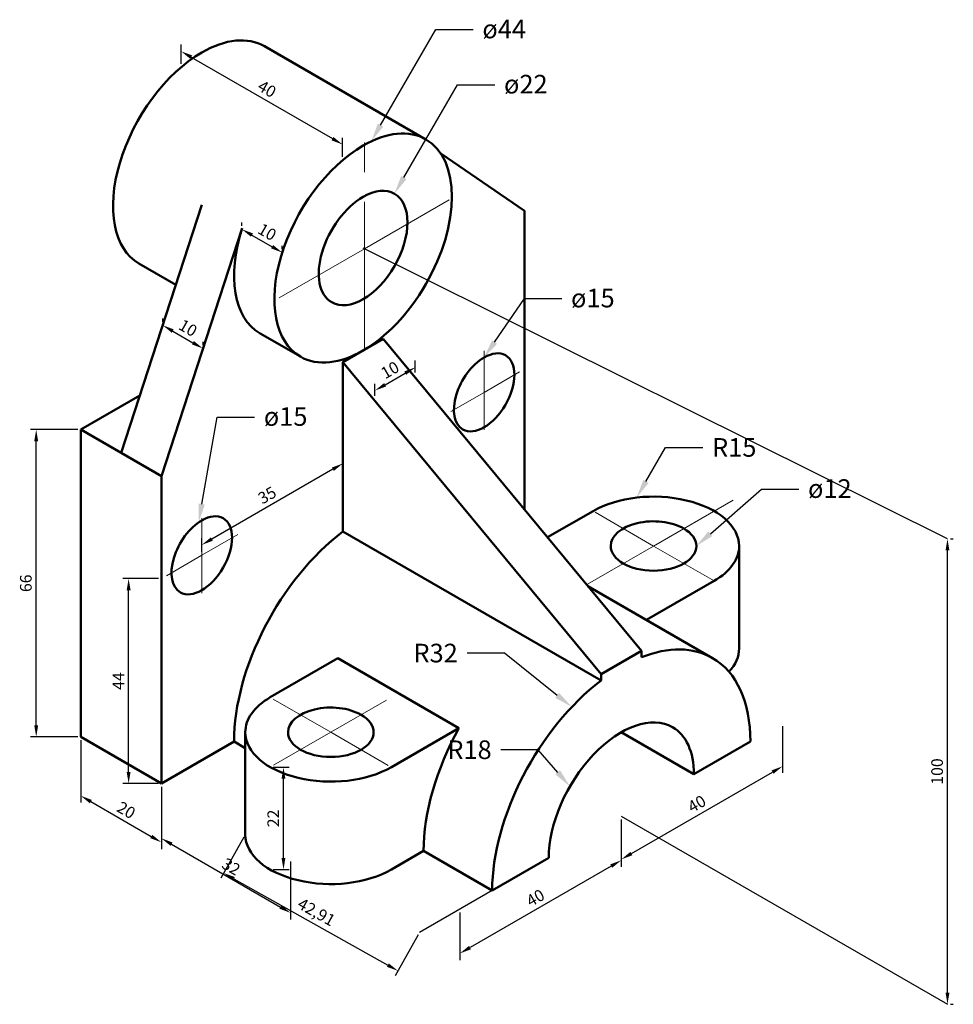
# Model space of a CAD drawing. Units: millimetres. Extents: x 3050 to 3251, y 1794 to 2006.
import ezdxf
from ezdxf import colors
from ezdxf.entities.mleader import LeaderData, LeaderLine
from ezdxf.math import Vec2, Vec3

# ---------------------------------------------------------------- set-up
doc = ezdxf.new("R2010")
doc.units = ezdxf.units.MM
doc.linetypes.add('CENTER', pattern=[50.8, 31.75, -6.35, 6.35, -6.35])
for name, color, linetype, lineweight in [('M-CNTR', 1, 'CENTER', 18), ('M-DIMS', 2, 'Continuous', 25), ('M-OUTL', 7, 'Continuous', 50), ('M-TEXT', 3, 'Continuous', 25)]:
    doc.layers.add(name, color=color, linetype=linetype, lineweight=lineweight)
doc.styles.get("Standard").update_dxf_attribs({"font": 'arial.ttf'})
doc.dimstyles.new('ISO-25', dxfattribs={"dimtxt": 2.5, "dimasz": 2.5, "dimexe": 1.25, "dimexo": 0.625, "dimtad": 1, "dimtxsty": 'Standard', "dimcen": 2.5, "dimadec": 0, "dimazin": 0, "dimtfac": 1, "dimtmove": 0, "dimatfit": 3, "dimfxl": 1, "dimarcsym": 0})

# ---------------------------------------------------------------- blocks, each defined once
blk = doc.blocks.new('*D1')
at = {"layer": 'Defpoints', "color": 0, "transparency": 16777216}
for p in [(3063.23, 1851.76), (3080.55, 1841.76), (3080.55, 1829.12)]:
    blk.add_point(p, dxfattribs=at)
at = {"layer": 'M-DIMS', "color": 0, "lineweight": -2, "transparency": 16777216}
for p, q in [((3063.23, 1851.04), (3063.23, 1837.67)), ((3080.55, 1841.04), (3080.55, 1827.67)), ((3065.39, 1837.87), (3078.38, 1830.37))]:
    blk.add_line(p, q, dxfattribs=at)
at = {"layer": 'M-DIMS', "color": 0, "transparency": 16777216}
for points in [[(3065.6, 1838.23), (3065.18, 1837.51), (3063.23, 1839.12)], [(3078.59, 1830.73), (3078.18, 1830.01), (3080.55, 1829.12)]]:
    blk.add_solid(points, dxfattribs=at)
at = {"layer": 'M-DIMS', "color": 0, "transparency": 16777216, "insert": (3072.84, 1835.76), "char_height": 2.5, "attachment_point": 5, "rotation": 330}
blk.add_mtext('20', dxfattribs=at)
blk = doc.blocks.new('*D2')
at = {"layer": 'Defpoints', "color": 0, "transparency": 16777216}
for p in [(3080.55, 1841.76), (3108.26, 1825.76), (3108.26, 1813.98)]:
    blk.add_point(p, dxfattribs=at)
at = {"layer": 'M-DIMS', "color": 0, "lineweight": -2, "transparency": 16777216}
for p, q in [((3080.55, 1841.04), (3080.55, 1828.54)), ((3082.71, 1828.73), (3106.1, 1815.23)), ((3108.26, 1825.04), (3108.26, 1812.54))]:
    blk.add_line(p, q, dxfattribs=at)
at = {"layer": 'M-DIMS', "color": 0, "transparency": 16777216}
for points in [[(3082.92, 1829.09), (3082.51, 1828.37), (3080.55, 1829.98)], [(3106.3, 1815.59), (3105.89, 1814.87), (3108.26, 1813.98)]]:
    blk.add_solid(points, dxfattribs=at)
at = {"layer": 'M-DIMS', "color": 0, "transparency": 16777216, "insert": (3095.36, 1823.63), "char_height": 2.5, "attachment_point": 5, "rotation": 330}
blk.add_mtext('32', dxfattribs=at)
blk = doc.blocks.new('*D3')
at = {"layer": 'Defpoints', "color": 0, "transparency": 16777216}
for p in [(3179.28, 1834.76), (3144.63, 1814.76), (3144.63, 1805.27)]:
    blk.add_point(p, dxfattribs=at)
at = {"layer": 'M-DIMS', "color": 0, "lineweight": -2, "transparency": 16777216}
for p, q in [((3179.28, 1834.04), (3179.28, 1823.83)), ((3177.11, 1824.02), (3146.8, 1806.52)), ((3144.63, 1814.04), (3144.63, 1803.83))]:
    blk.add_line(p, q, dxfattribs=at)
at = {"layer": 'M-DIMS', "color": 0, "transparency": 16777216}
for points in [[(3176.9, 1824.38), (3177.32, 1823.66), (3179.28, 1825.27)], [(3146.59, 1806.88), (3147.01, 1806.16), (3144.63, 1805.27)]]:
    blk.add_solid(points, dxfattribs=at)
at = {"layer": 'M-DIMS', "color": 0, "transparency": 16777216, "insert": (3161, 1816.92), "char_height": 2.5, "attachment_point": 5, "rotation": 30}
blk.add_mtext('40', dxfattribs=at)
blk = doc.blocks.new('*D4')
at = {"layer": 'Defpoints', "color": 0, "transparency": 16777216}
for p in [(3213.92, 1854.76), (3213.92, 1845.46), (3179.28, 1834.76)]:
    blk.add_point(p, dxfattribs=at)
at = {"layer": 'M-DIMS', "color": 0, "lineweight": -2, "transparency": 16777216}
for p, q in [((3213.92, 1854.04), (3213.92, 1844.02)), ((3181.44, 1826.71), (3211.75, 1844.21)), ((3179.28, 1834.04), (3179.28, 1824.02))]:
    blk.add_line(p, q, dxfattribs=at)
at = {"layer": 'M-DIMS', "color": 0, "transparency": 16777216}
for points in [[(3211.54, 1844.57), (3211.96, 1843.85), (3213.92, 1845.46)], [(3181.23, 1827.07), (3181.65, 1826.35), (3179.28, 1825.46)]]:
    blk.add_solid(points, dxfattribs=at)
at = {"layer": 'M-DIMS', "color": 0, "transparency": 16777216, "insert": (3195.65, 1837.11), "char_height": 2.5, "attachment_point": 5, "rotation": 30}
blk.add_mtext('40', dxfattribs=at)
blk = doc.blocks.new('*D5')
at = {"layer": 'Defpoints', "color": 0, "transparency": 16777216}
for p in [(3053.67, 1917.76), (3063.23, 1917.76), (3063.23, 1851.76)]:
    blk.add_point(p, dxfattribs=at)
at = {"layer": 'M-DIMS', "color": 0, "lineweight": -2, "transparency": 16777216}
for p, q in [((3062.6, 1917.76), (3052.42, 1917.76)), ((3053.67, 1854.26), (3053.67, 1915.26)), ((3062.6, 1851.76), (3052.42, 1851.76))]:
    blk.add_line(p, q, dxfattribs=at)
at = {"layer": 'M-DIMS', "color": 0, "transparency": 16777216}
for points in [[(3053.25, 1915.26), (3054.09, 1915.26), (3053.67, 1917.76)], [(3053.25, 1854.26), (3054.09, 1854.26), (3053.67, 1851.76)]]:
    blk.add_solid(points, dxfattribs=at)
at = {"layer": 'M-DIMS', "color": 0, "transparency": 16777216, "insert": (3051.77, 1884.76), "char_height": 2.5, "attachment_point": 5, "rotation": 90}
blk.add_mtext('66', dxfattribs=at)
blk = doc.blocks.new('*D6')
at = {"layer": 'Defpoints', "color": 0, "transparency": 16777216}
for p in [(3073.51, 1885.76), (3080.55, 1885.76), (3080.55, 1841.76)]:
    blk.add_point(p, dxfattribs=at)
at = {"layer": 'M-DIMS', "color": 0, "lineweight": -2, "transparency": 16777216}
for p, q in [((3079.92, 1885.76), (3072.26, 1885.76)), ((3073.51, 1844.26), (3073.51, 1883.26)), ((3079.92, 1841.76), (3072.26, 1841.76))]:
    blk.add_line(p, q, dxfattribs=at)
at = {"layer": 'M-DIMS', "color": 0, "transparency": 16777216}
for points in [[(3073.09, 1883.26), (3073.93, 1883.26), (3073.51, 1885.76)], [(3073.09, 1844.26), (3073.93, 1844.26), (3073.51, 1841.76)]]:
    blk.add_solid(points, dxfattribs=at)
at = {"layer": 'M-DIMS', "color": 0, "transparency": 16777216, "insert": (3071.64, 1863.76), "char_height": 2.5, "attachment_point": 5, "rotation": 90}
blk.add_mtext('44', dxfattribs=at)
blk = doc.blocks.new('*D7')
at = {"layer": 'Defpoints', "color": 0, "transparency": 16777216}
for p in [(3119.52, 1908.26), (3089.21, 1893), (3089.21, 1890.76)]:
    blk.add_point(p, dxfattribs=at)
at = {"layer": 'M-DIMS', "color": 0, "lineweight": -2, "transparency": 16777216}
for p, q in [((3119.52, 1908.99), (3119.52, 1911.95)), ((3117.35, 1909.25), (3091.37, 1894.25)), ((3089.21, 1891.49), (3089.21, 1894.45))]:
    blk.add_line(p, q, dxfattribs=at)
at = {"layer": 'M-DIMS', "color": 0, "transparency": 16777216}
for points in [[(3117.15, 1909.61), (3117.56, 1908.89), (3119.52, 1910.5)], [(3091.17, 1894.61), (3091.58, 1893.89), (3089.21, 1893)]]:
    blk.add_solid(points, dxfattribs=at)
at = {"layer": 'M-DIMS', "color": 0, "transparency": 16777216, "insert": (3103.41, 1903.4), "char_height": 2.5, "attachment_point": 5, "rotation": 30}
blk.add_mtext('35', dxfattribs=at)
blk = doc.blocks.new('*D8')
at = {"layer": 'Defpoints', "color": 0, "transparency": 16777216}
for p in [(3135.06, 1931.15), (3135.06, 1929.33), (3126.4, 1924.33)]:
    blk.add_point(p, dxfattribs=at)
at = {"layer": 'M-DIMS', "color": 0, "lineweight": -2, "transparency": 16777216}
for p, q in [((3135.06, 1930.05), (3135.06, 1932.59)), ((3128.57, 1927.4), (3132.9, 1929.9)), ((3126.4, 1925.05), (3126.4, 1927.59))]:
    blk.add_line(p, q, dxfattribs=at)
at = {"layer": 'M-DIMS', "color": 0, "transparency": 16777216}
for points in [[(3132.69, 1930.26), (3133.1, 1929.53), (3135.06, 1931.15)], [(3128.36, 1927.76), (3128.77, 1927.03), (3126.4, 1926.15)]]:
    blk.add_solid(points, dxfattribs=at)
at = {"layer": 'M-DIMS', "color": 0, "transparency": 16777216, "insert": (3129.78, 1930.29), "char_height": 2.5, "attachment_point": 5, "rotation": 30}
blk.add_mtext('10', dxfattribs=at)
blk = doc.blocks.new('*D9')
at = {"layer": 'Defpoints', "color": 0, "transparency": 16777216}
for p in [(3103.93, 1845.26), (3106.76, 1845.26), (3103.93, 1823.26)]:
    blk.add_point(p, dxfattribs=at)
at = {"layer": 'M-DIMS', "color": 0, "lineweight": -2, "transparency": 16777216}
for p, q in [((3104.56, 1845.26), (3108.01, 1845.26)), ((3106.76, 1825.76), (3106.76, 1842.76)), ((3104.56, 1823.26), (3108.01, 1823.26))]:
    blk.add_line(p, q, dxfattribs=at)
at = {"layer": 'M-DIMS', "color": 0, "transparency": 16777216}
for points in [[(3106.34, 1842.76), (3107.17, 1842.76), (3106.76, 1845.26)], [(3106.34, 1825.76), (3107.17, 1825.76), (3106.76, 1823.26)]]:
    blk.add_solid(points, dxfattribs=at)
at = {"layer": 'M-DIMS', "color": 0, "transparency": 16777216, "insert": (3104.88, 1834.26), "char_height": 2.5, "attachment_point": 5, "rotation": 90}
blk.add_mtext('22', dxfattribs=at)
blk = doc.blocks.new('*D10')
at = {"layer": 'Defpoints', "color": 0, "transparency": 16777216}
for p in [(3080.82, 1940.18), (3089.48, 1935.18), (3089.48, 1935.18)]:
    blk.add_point(p, dxfattribs=at)
at = {"layer": 'M-DIMS', "color": 0, "lineweight": -2, "transparency": 16777216}
for p, q in [((3080.82, 1940.9), (3080.82, 1941.62)), ((3082.98, 1938.93), (3087.31, 1936.43)), ((3089.48, 1935.9), (3089.48, 1936.62))]:
    blk.add_line(p, q, dxfattribs=at)
at = {"layer": 'M-DIMS', "color": 0, "transparency": 16777216}
for points in [[(3083.19, 1939.29), (3082.78, 1938.56), (3080.82, 1940.18)], [(3087.52, 1936.79), (3087.11, 1936.06), (3089.48, 1935.18)]]:
    blk.add_solid(points, dxfattribs=at)
at = {"layer": 'M-DIMS', "color": 0, "transparency": 16777216, "insert": (3086.1, 1939.32), "char_height": 2.5, "attachment_point": 5, "rotation": 330}
blk.add_mtext('10', dxfattribs=at)
blk = doc.blocks.new('*D11')
at = {"layer": 'Defpoints', "color": 0, "transparency": 16777216}
for p in [(3097.82, 1960.79), (3106.48, 1955.79), (3106.48, 1955.79)]:
    blk.add_point(p, dxfattribs=at)
at = {"layer": 'M-DIMS', "color": 0, "lineweight": -2, "transparency": 16777216}
for p, q in [((3097.82, 1961.51), (3097.82, 1962.23)), ((3099.99, 1959.54), (3104.32, 1957.04)), ((3106.48, 1956.51), (3106.48, 1957.23))]:
    blk.add_line(p, q, dxfattribs=at)
at = {"layer": 'M-DIMS', "color": 0, "transparency": 16777216}
for points in [[(3100.2, 1959.9), (3099.78, 1959.18), (3097.82, 1960.79)], [(3104.53, 1957.4), (3104.11, 1956.68), (3106.48, 1955.79)]]:
    blk.add_solid(points, dxfattribs=at)
at = {"layer": 'M-DIMS', "color": 0, "transparency": 16777216, "insert": (3103.1, 1959.93), "char_height": 2.5, "attachment_point": 5, "rotation": 330}
blk.add_mtext('10', dxfattribs=at)
blk = doc.blocks.new('*D12')
at = {"layer": 'Defpoints', "color": 0, "transparency": 16777216}
for p in [(3084.79, 1995.61), (3119.43, 1979), (3119.43, 1975.61)]:
    blk.add_point(p, dxfattribs=at)
at = {"layer": 'M-DIMS', "color": 0, "lineweight": -2, "transparency": 16777216}
for p, q in [((3084.79, 1996.34), (3084.79, 2000.45)), ((3086.95, 1997.75), (3117.27, 1980.25)), ((3119.43, 1976.34), (3119.43, 1980.45))]:
    blk.add_line(p, q, dxfattribs=at)
at = {"layer": 'M-DIMS', "color": 0, "transparency": 16777216}
for points in [[(3087.16, 1998.12), (3086.75, 1997.39), (3084.79, 1999)], [(3117.47, 1980.62), (3117.06, 1979.89), (3119.43, 1979)]]:
    blk.add_solid(points, dxfattribs=at)
at = {"layer": 'M-DIMS', "color": 0, "transparency": 16777216, "insert": (3103.06, 1990.65), "char_height": 2.5, "attachment_point": 5, "rotation": 330}
blk.add_mtext('40', dxfattribs=at)
blk = doc.blocks.new('*D13')
at = {"layer": 'Defpoints', "color": 0, "transparency": 16777216}
for p in [(3098.55, 1830.76), (3135.97, 1809.76), (3131.35, 1801.52)]:
    blk.add_point(p, dxfattribs=at)
at = {"layer": 'M-DIMS', "color": 0, "lineweight": -2, "transparency": 16777216}
for p, q in [((3098.24, 1830.22), (3093.32, 1821.43)), ((3096.11, 1821.3), (3129.17, 1802.75)), ((3135.67, 1809.22), (3130.74, 1800.43))]:
    blk.add_line(p, q, dxfattribs=at)
at = {"layer": 'M-DIMS', "color": 0, "transparency": 16777216}
for points in [[(3096.31, 1821.66), (3095.9, 1820.94), (3093.93, 1822.52)], [(3129.37, 1803.11), (3128.97, 1802.38), (3131.35, 1801.52)]]:
    blk.add_solid(points, dxfattribs=at)
at = {"layer": 'M-DIMS', "color": 0, "transparency": 16777216, "insert": (3113.68, 1813.88), "char_height": 2.5, "attachment_point": 5, "rotation": 330.7014}
blk.add_mtext('42,91', dxfattribs=at)
blk = doc.blocks.new('*D14')
at = {"layer": 'Defpoints', "color": 0, "transparency": 16777216}
for p in [(3249.3, 1894.33), (3249.3, 1894.33), (3249.3, 1794.33)]:
    blk.add_point(p, dxfattribs=at)
at = {"layer": 'M-DIMS', "color": 0, "lineweight": -2, "transparency": 16777216}
for p, q in [((3249.93, 1894.33), (3250.55, 1894.33)), ((3249.3, 1796.83), (3249.3, 1891.83)), ((3249.93, 1794.33), (3250.55, 1794.33))]:
    blk.add_line(p, q, dxfattribs=at)
at = {"layer": 'M-DIMS', "color": 0, "transparency": 16777216}
for points in [[(3248.89, 1891.83), (3249.72, 1891.83), (3249.3, 1894.33)], [(3248.89, 1796.83), (3249.72, 1796.83), (3249.3, 1794.33)]]:
    blk.add_solid(points, dxfattribs=at)
at = {"layer": 'M-DIMS', "color": 0, "transparency": 16777216, "insert": (3247.4, 1844.33), "char_height": 2.5, "attachment_point": 5, "rotation": 90}
blk.add_mtext('100', dxfattribs=at)

msp = doc.modelspace()

# ---------------------------------------------------------------- linework, layer by layer
at = {"layer": 'M-CNTR'}
for p, q in [((3124.166, 1934.95), (3124.166, 1979.681)), ((3124.166, 1956.608), (3142.356, 1967.11)), ((3124.166, 1956.608), (3105.843, 1946.029)), ((3149.831, 1925.765), (3149.831, 1934.653)), ((3149.831, 1925.765), (3157.41, 1930.141)), ((3149.831, 1925.765), (3142.7, 1921.648)), ((3149.831, 1925.765), (3149.831, 1917.715)), ((3186.204, 1892.765), (3203.267, 1902.616)), ((3186.204, 1892.765), (3173.653, 1900.011)), ((3089.209, 1890.765), (3089.209, 1898.721)), ((3089.209, 1890.765), (3096.935, 1895.225)), ((3186.204, 1892.765), (3172.045, 1884.59)), ((3186.204, 1892.765), (3199.194, 1885.265)), ((3089.209, 1890.765), (3081.622, 1886.384)), ((3089.209, 1890.765), (3089.209, 1882.603)), ((3116.922, 1852.765), (3104.573, 1859.894)), ((3116.922, 1852.765), (3128.866, 1859.661)), ((3116.922, 1852.765), (3104.649, 1845.679)), ((3116.922, 1852.765), (3129.25, 1845.647))]:
    msp.add_line(p, q, dxfattribs=at)
at = {"layer": 'M-DIMS'}
for p, q in [((3249.303, 1894.335), (3123.85, 1956.765)), ((3179.276, 1834.765), (3223.608, 1809.169)), ((3151.563, 1818.765), (3135.974, 1809.765)), ((3223.608, 1809.169), (3249.303, 1794.335))]:
    msp.add_line(p, q, dxfattribs=at)
at = {"layer": 'M-OUTL'}
for p, q in [((3102.681, 2000.099), (3102.681, 2000.099)), ((3137.322, 1980.099), (3102.681, 2000.099)), ((3158.491, 1964.765), (3140.529, 1977.028)), ((3071.888, 1912.765), (3089.242, 1966.033)), ((3158.491, 1900.624), (3158.491, 1964.765)), ((3080.549, 1907.765), (3097.903, 1961.033)), ((3083.649, 1948.862), (3075.737, 1953.43)), ((3110.378, 1933.43), (3101.718, 1938.43)), ((3119.52, 1932.265), (3128.18, 1937.265)), ((3183.606, 1870.265), (3128.18, 1937.265)), ((3119.52, 1932.265), (3119.52, 1895.872)), ((3174.946, 1865.265), (3119.52, 1932.265)), ((3063.228, 1917.765), (3075.901, 1925.081)), ((3071.888, 1912.765), (3063.228, 1917.765)), ((3063.228, 1851.765), (3063.228, 1917.765)), ((3080.549, 1907.765), (3071.888, 1912.765)), ((3080.549, 1841.765), (3080.549, 1907.765)), ((3163.451, 1894.628), (3173.213, 1900.265)), ((3174.946, 1863.872), (3119.52, 1895.872)), ((3204.575, 1870.765), (3204.575, 1892.765)), ((3184.692, 1876.892), (3199.194, 1885.265)), ((3198.872, 1868.706), (3172.117, 1884.153)), ((3174.946, 1865.265), (3183.606, 1870.265)), ((3183.606, 1868.872), (3183.606, 1870.265)), ((3103.931, 1860.265), (3118.448, 1868.646)), ((3144.429, 1853.646), (3118.448, 1868.646)), ((3174.946, 1863.872), (3174.946, 1865.265)), ((3098.551, 1830.765), (3098.551, 1852.765)), ((3129.912, 1845.265), (3144.429, 1853.646)), ((3194.864, 1843.765), (3179.276, 1852.765)), ((3080.549, 1841.765), (3063.228, 1851.765)), ((3080.549, 1841.765), (3096.137, 1850.765)), ((3098.551, 1849.371), (3096.137, 1850.765)), ((3194.864, 1843.765), (3206.988, 1850.765)), ((3129.912, 1823.265), (3136.84, 1827.265)), ((3151.563, 1818.765), (3136.84, 1827.265)), ((3151.563, 1818.765), (3163.687, 1825.765)), ((3103.931, 1823.265), (3103.931, 1823.265))]:
    msp.add_line(p, q, dxfattribs=at)
for centre, major_axis, start_param, end_param in [((3089.209, 1976.765), (13.472, 23.335), 0, 0.7853982), ((3089.209, 1976.765), (13.472, 23.335), 0.7853982, 3.1415927), ((3123.85, 1956.765), (13.472, 23.335), 0, 0.7853982), ((3123.85, 1956.765), (13.472, 23.335), 3.1415927, 6.2831853), ((3123.85, 1956.765), (13.472, 23.335), 0.7853982, 3.1415927), ((3123.85, 1956.765), (6.736, 11.667), 0, 0.7853982), ((3123.85, 1956.765), (6.736, 11.667), 0.7853982, 3.1415927), ((3123.85, 1956.765), (6.736, 11.667), 3.1415927, 6.2831853), ((3115.19, 1961.765), (13.472, 23.335), 1.9223093, 3.1415927), ((3149.831, 1925.765), (4.593, 7.955), 0.7853982, 3.1415927), ((3149.831, 1925.765), (4.593, 7.955), 3.1415927, 6.2831853), ((3149.831, 1925.765), (4.593, 7.955), 0, 0.7853982), ((3186.204, 1892.765), (18.371, 0), 0, 2.3561945), ((3089.209, 1890.765), (4.593, 7.955), 0, 0.7853982), ((3089.209, 1890.765), (4.593, 7.955), 0.7853982, 3.1415927), ((3089.209, 1890.765), (4.593, 7.955), 3.1415927, 6.2831853), ((3186.204, 1892.765), (9.186, 0), 0.7853982, 3.1415927), ((3123.85, 1866.765), (19.596, 33.941), 0.942291, 2.3561945), ((3186.204, 1892.765), (9.186, 0), 0, 0.7853982), ((3186.204, 1892.765), (9.186, 0), 3.1415927, 6.2831853), ((3186.204, 1892.765), (18.371, 0), 5.4977871, 6.2831853), ((3179.276, 1834.765), (19.596, 33.941), 0, 0.6285053), ((3186.204, 1870.765), (-18.371, 0), 2.6496796, 3.1415927), ((3179.276, 1834.765), (19.596, 33.941), 5.4977871, 6.2831853), ((3179.276, 1834.765), (19.596, 33.941), 0.942291, 2.3561945), ((3116.922, 1852.765), (18.371, 0), 2.3561945, 3.1415927), ((3116.922, 1852.765), (9.186, 0), 0.7853982, 3.1415927), ((3116.922, 1852.765), (9.186, 0), 0, 0.7853982), ((3179.276, 1834.765), (11.023, 19.092), 0, 2.3561945), ((3116.922, 1852.765), (18.371, 0), 3.1415927, 5.4977871), ((3116.922, 1852.765), (9.186, 0), 3.1415927, 6.2831853), ((3164.553, 1843.265), (19.596, 33.941), 1.5981537, 2.3561945), ((3179.276, 1834.765), (11.023, 19.092), 5.4977871, 6.2831853), ((3116.922, 1830.765), (18.371, 0), 3.1415927, 5.4977871)]:
    msp.add_ellipse(centre, major_axis=major_axis, ratio=0.5773503, start_param=start_param, end_param=end_param, dxfattribs=at)

# ---------------------------------------------------------------- dimensions: what is measured, and where the dimension line sits
at = {"layer": 'M-DIMS'}
for p1, p2, distance, picture, middle in [((3084.79, 1995.613), (3119.431, 1975.613), 2.937, '*D12', (3103.061, 1990.651)), ((3097.823, 1960.786), (3106.483, 1955.786), 0, '*D11', (3103.104, 1959.933)), ((3080.818, 1940.175), (3089.479, 1935.175), 0, '*D10', (3086.099, 1939.322)), ((3126.4, 1924.328), (3135.06, 1929.328), 1.574, '*D8', (3129.78, 1930.292)), ((3063.228, 1851.765), (3063.228, 1917.765), 9.559, '*D5', (3051.768, 1884.765)), ((3119.52, 1908.265), (3089.209, 1890.765), -1.938, '*D7', (3103.413, 1903.4)), ((3080.549, 1841.765), (3080.549, 1885.765), 7.038, '*D6', (3071.636, 1863.765)), ((3179.276, 1834.765), (3213.917, 1854.765), -8.056, '*D4', (3195.645, 1837.109)), ((3063.228, 1851.765), (3080.549, 1841.765), -10.953, '*D1', (3072.839, 1835.764)), ((3103.931, 1823.265), (3103.931, 1845.265), -2.824, '*D9', (3104.876, 1834.265)), ((3080.549, 1841.765), (3108.262, 1825.765), -10.205, '*D2', (3095.356, 1823.629)), ((3179.276, 1834.765), (3144.635, 1814.765), 8.221, '*D3', (3161.004, 1816.919))]:
    dim = msp.add_aligned_dim(p1=p1, p2=p2, distance=distance, dimstyle='ISO-25', override={"dimclrd": 0, "dimclre": 0, "dimclrt": 0}, dxfattribs=at)
    dim.commit()
    dim.dimension.update_dxf_attribs({"geometry": picture, "text_midpoint": middle})
for base, p1, p2, angle, picture, middle in [((3249.303, 1894.335), (3249.303, 1794.335), (3249.303, 1894.335), 90, '*D14', (3247.401, 1844.335)), ((3131.351, 1801.525), (3098.551, 1830.765), (3135.974, 1809.765), 330.70141, '*D13', (3113.68, 1813.88))]:
    dim = msp.add_linear_dim(base=base, p1=p1, p2=p2, angle=angle, dimstyle='ISO-25', override={"dimrnd": 0}, dxfattribs=at)
    dim.commit()
    dim.dimension.update_dxf_attribs({"geometry": picture, "text_midpoint": middle})

# ---------------------------------------------------------------- leaders
at = {"layer": 'M-TEXT'}
ml = msp.add_multileader_mtext('Standard', dxfattribs=at)
ml.set_content('ø44', color=256)
ml.set_leader_properties()
ml.build(insert=Vec2(0, 0))
ctx = ml.context
ctx.base_point, ctx.plane_origin = Vec3(3147.46, 2003.693), Vec3(3125.597, 1979.681)
notes = []
notes.append((ctx, [(0, (1, 1, 0), (3139.46, 2003.693), (1, 0), 8, [(0, [(3125.597, 1979.681)], 0, [])])]))
ctx.mtext.insert, ctx.mtext.flow_direction = Vec3(3149.46, 2005.801), 5
ml = msp.add_multileader_mtext('Standard', dxfattribs=at)
ml.set_content('ø22', color=256)
ml.set_leader_properties()
ml.build(insert=Vec2(0, 0))
ctx = ml.context
ctx.base_point, ctx.plane_origin = Vec3(3152.103, 1991.844), Vec3(3130.586, 1968.432)
notes.append((ctx, [(0, (1, 1, 0), (3144.103, 1991.844), (1, 0), 8, [(0, [(3130.586, 1968.432)], 0, [])])]))
ctx.mtext.insert, ctx.mtext.flow_direction = Vec3(3154.103, 1993.951), 5
ml = msp.add_multileader_mtext('Standard', dxfattribs=at)
ml.set_content('ø15', color=256)
ml.set_leader_properties()
ml.build(insert=Vec2(0, 0))
ctx = ml.context
ctx.base_point, ctx.plane_origin = Vec3(3166.491, 1945.906), Vec3(3149.806, 1933.25)
notes.append((ctx, [(0, (1, 1, 0), (3158.491, 1945.906), (1, 0), 8, [(0, [(3149.806, 1933.25)], 0, [])])]))
ctx.mtext.insert, ctx.mtext.flow_direction = Vec3(3168.491, 1948.014), 5
ml = msp.add_multileader_mtext('Standard', dxfattribs=at)
ml.set_content('ø15', color=256)
ml.set_leader_properties()
ml.build(insert=Vec2(0, 0))
ctx = ml.context
ctx.base_point, ctx.plane_origin = Vec3(3100.54, 1920.469), Vec3(3088.533, 1897.834)
notes.append((ctx, [(0, (1, 1, 0), (3092.54, 1920.469), (1, 0), 8, [(0, [(3088.533, 1897.834)], 0, [])])]))
ctx.mtext.insert, ctx.mtext.flow_direction = Vec3(3102.54, 1922.577), 5
ml = msp.add_multileader_mtext('Standard', dxfattribs=at)
ml.set_content('R15', color=256)
ml.set_leader_properties()
ml.build(insert=Vec2(0, 0))
ctx = ml.context
ctx.base_point, ctx.plane_origin = Vec3(3196.766, 1913.899), Vec3(3182.566, 1903.161)
notes.append((ctx, [(0, (1, 1, 0), (3188.766, 1913.899), (1, 0), 8, [(0, [(3182.566, 1903.161)], 0, [])])]))
ctx.mtext.insert, ctx.mtext.flow_direction = Vec3(3198.766, 1915.934), 5
ml = msp.add_multileader_mtext('Standard', dxfattribs=at)
ml.set_content('ø12', color=256)
ml.set_leader_properties()
ml.build(insert=Vec2(0, 0))
ctx = ml.context
ctx.base_point, ctx.plane_origin = Vec3(3217.37, 1904.988), Vec3(3195.389, 1892.765)
notes.append((ctx, [(0, (1, 1, 0), (3209.37, 1904.988), (1, 0), 8, [(0, [(3195.389, 1892.765)], 0, [])])]))
ctx.mtext.insert, ctx.mtext.flow_direction = Vec3(3219.37, 1907.096), 5
ml = msp.add_multileader_mtext('Standard', dxfattribs=at)
ml.set_content('R32', color=256)
ml.set_leader_properties()
ml.build(insert=Vec2(0, 0))
ctx = ml.context
ctx.base_point, ctx.plane_origin = Vec3(3132.659, 1869.732), Vec3(3168.653, 1858.188)
ctx.text_align_type = 2
notes.append((ctx, [(0, (1, 1, 0), (3154.176, 1869.732), (-1, 0), 8, [(0, [(3168.653, 1858.188)], 0, [])])]))
ctx.mtext.insert, ctx.mtext.alignment, ctx.mtext.flow_direction = Vec3(3144.176, 1871.768), 3, 5
ml = msp.add_multileader_mtext('Standard', dxfattribs=at)
ml.set_content('R18', color=256)
ml.set_leader_properties()
ml.build(insert=Vec2(0, 0))
ctx = ml.context
ctx.base_point, ctx.plane_origin = Vec3(3139.884, 1848.976), Vec3(3168.253, 1841.129)
ctx.text_align_type = 2
notes.append((ctx, [(0, (1, 1, 0), (3161.451, 1848.976), (-1, 0), 8, [(0, [(3168.253, 1841.129)], 0, [])])]))
ctx.mtext.insert, ctx.mtext.alignment, ctx.mtext.flow_direction = Vec3(3151.451, 1851.01), 3, 5
for ctx, leaders in notes:
    for number, flags, end, landing, length, lines in leaders:
        leader = LeaderData()
        leader.index, (leader.has_last_leader_line, leader.has_dogleg_vector, leader.attachment_direction) = number, flags
        leader.last_leader_point, leader.dogleg_vector, leader.dogleg_length = Vec3(end), Vec3(landing), length
        for number, points, colour, breaks in lines:
            line = LeaderLine()
            line.index, line.vertices, line.color, line.breaks = number, Vec3.list(points), colors.encode_raw_color(colour), breaks
            leader.lines.append(line)
        ctx.leaders.append(leader)

doc.saveas('drawing.dxf')
